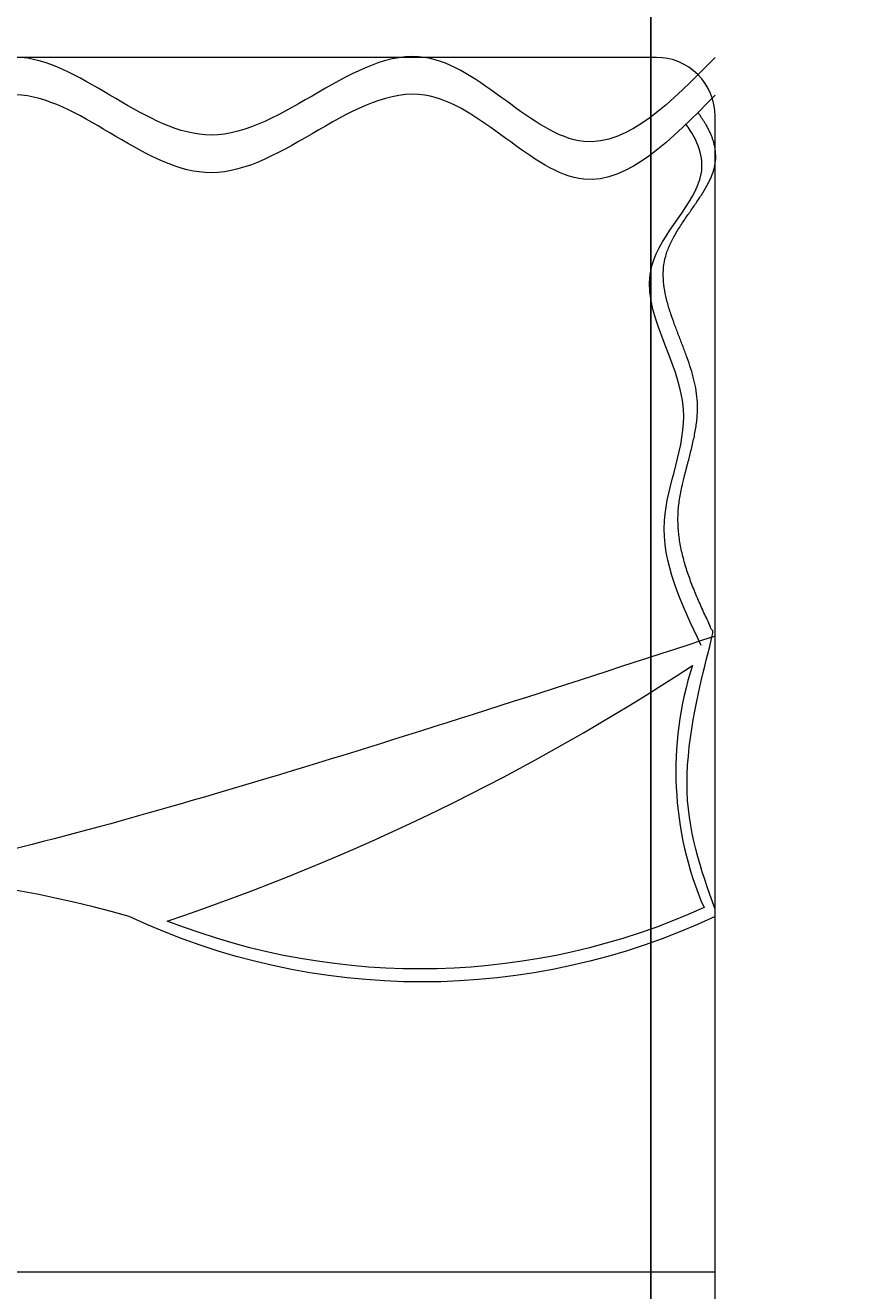
# Model space of a CAD drawing. Units: inches. Extents: x -61 to 1599, y -1316 to 257.
# Tile 53 of 204: x 143 to 192, y -408 to -334. Entities that reach past the tile are written whole.
import ezdxf

# ---------------------------------------------------------------- set-up
doc = ezdxf.new("R2010")
doc.units = ezdxf.units.IN
doc.header["$MEASUREMENT"] = 0
doc.layers.add('A-ANNO-DIMS', color=2, linetype='Continuous', lineweight=18)
doc.layers.add('FURNITURE', color=83, linetype='Continuous', lineweight=18)
doc.styles.get("Standard").update_dxf_attribs({"font": 'arial.ttf'})
doc.dimstyles.get("Standard").update_dxf_attribs({"dimtxt": 0.18, "dimasz": 0.18, "dimexe": 0.18, "dimexo": 0.0625, "dimgap": 0.09, "dimtad": 0, "dimtih": 1, "dimtoh": 1, "dimdec": 0, "dimzin": 0, "dimdsep": 46, "dimlunit": 3, "dimtxsty": 'Standard', "dimcen": 0.09, "dimadec": 0, "dimazin": 0, "dimtfac": 1, "dimtdec": 0, "dimtofl": 0, "dimtmove": 0, "dimatfit": 3, "dimfxl": 1, "dimtolj": 1, "dimtzin": 0, "dimarcsym": 0})

# ---------------------------------------------------------------- blocks, each defined once
blk = doc.blocks.new('BED-DOUBLE')
blk.add_line((1.272, 20.467), (70.263, 20.467))
for points in [[(1.272, 88.537), (1.272, 3.449, 0.414214), (4.722, 0), (66.813, 0, 0.414214), (70.263, 3.449), (70.263, 88.537, 0.414214), (66.813, 91.987), (4.722, 91.987, 0.414214)], [(38.01, 41.126, 0.064396), (68.933, 56.181, 0.181766), (69.614, 41.916, -0.202767)]]:
    blk.add_lwpolyline(points, format="xyb", close=True)
blk.add_lwpolyline([(70.263, 41.387, -0.22309), (35.767, 41.387, 0.142156), (1.272, 41.387)], format="xyb")
for points, knots in [([(70.263, 91.987), (67.707, 89.379), (62.206, 83.764), (52.487, 96.724), (40.92, 82.741), (28.609, 96.737), (15.695, 81.527), (6.205, 88.409), (1.272, 91.987)], [0, 0, 0, 0, 9.176033, 19.753992, 33.150145, 45.209422, 59.881559, 75.764594, 75.764594, 75.764594, 75.764594]), ([(70.263, 89.765), (67.707, 87.157), (62.206, 81.542), (52.487, 94.502), (40.92, 80.519), (28.609, 94.515), (15.695, 79.305), (6.205, 86.187), (1.272, 89.765)], [0, 0, 0, 0, 9.176033, 19.753992, 33.150145, 45.209422, 59.881559, 75.764594, 75.764594, 75.764594, 75.764594]), ([(69.451, 57.362), (68.289, 59.79), (66.113, 64.336), (70.043, 71.905), (64.118, 79.112), (70.314, 84.4), (69.244, 87.088), (68.552, 88.052)], [0, 0, 0, 0, 6.649676, 12.451782, 19.973966, 25.324174, 28.349676, 28.349676, 28.349676, 28.349676])]:
    blk.add_open_spline(points, degree=3, knots=knots)
for points, weights, knots in [([(70.263, 41.825), (68.018, 47.029), (68.018, 52.696), (70.263, 57.9), (69.1, 60.328), (66.924, 64.874), (70.854, 72.444), (64.929, 79.65), (71.186, 84.991), (70.014, 87.727), (69.253, 88.741)], [1, 0.945466318698, 0.945466318698, 1, 1, 1, 1, 1, 1, 1, 1], [0, 0, 0, 0, 0.814571, 0.814571, 0.814571, 7.464247, 13.266353, 20.788537, 26.138745, 29.321895, 29.321895, 29.321895, 29.321895]), ([(70.263, 57.9), (59.862, 50.943), (48.595, 45.5), (36.681, 41.677), (36.463, 41.771), (36.247, 41.868), (36.032, 41.966), (24.597, 45.284), (12.692, 45.258), (1.272, 41.889), (2.723, 44.9), (5.745, 51.172), (0.137, 60.702), (6.828, 69.972), (0.109, 77.787), (4.354, 84.383), (5.398, 86.876)], [1, 0.993520320424, 0.993520320424, 1, 0.99997444972, 0.99997444972, 1, 0.973174868659, 0.973174868659, 1, 1, 1, 1, 1, 1, 1, 1], [0, 0, 0, 0, 0.279074, 0.279074, 0.279074, 0.296584, 0.296584, 0.296584, 0.865868, 0.865868, 0.865868, 9.142578, 18.107734, 25.769226, 34.110801, 40.441511, 40.441511, 40.441511, 40.441511])]:
    blk.add_rational_spline(points, weights, degree=3, knots=knots)
blk = doc.blocks.new('*D687')
at = {"layer": 'A-ANNO-DIMS', "color": 0, "lineweight": -2, "transparency": 16777216}
for p, q in [((289.418, 181.677), (-61.077, 181.677)), ((-60.897, 181.497), (-60.897, -528.952)), ((-60.897, -1239.765), (-60.897, -529.316)), ((319.64, -1239.945), (-61.077, -1239.945))]:
    blk.add_line(p, q, dxfattribs=at)
at = {"layer": 'A-ANNO-DIMS', "color": 0, "transparency": 16777216}
for points in [[(-60.927, 181.497), (-60.867, 181.497), (-60.897, 181.677)], [(-60.927, -1239.765), (-60.867, -1239.765), (-60.897, -1239.945)]]:
    blk.add_solid(points, dxfattribs=at)
at = {"layer": 'DEFPOINTS', "color": 0, "transparency": 16777216}
for p in [(289.481, 181.677), (-60.897, -1239.945), (319.703, -1239.945)]:
    blk.add_point(p, dxfattribs=at)
at = {"layer": 'A-ANNO-DIMS', "color": 0, "transparency": 16777216, "insert": (-60.897, -529.134), "char_height": 0.18, "attachment_point": 5}
blk.add_mtext('\\A1;1421.6', dxfattribs=at)
blk = doc.blocks.new('*D699')
at = {"layer": 'A-ANNO-DIMS', "color": 0, "lineweight": -2, "transparency": 16777216}
for p, q in [((835.64, -167.169), (-61.077, -167.169)), ((-60.897, -167.349), (-60.897, -306.726)), ((-60.897, -446.466), (-60.897, -307.09)), ((841.64, -446.646), (-61.077, -446.646))]:
    blk.add_line(p, q, dxfattribs=at)
at = {"layer": 'A-ANNO-DIMS', "color": 0, "transparency": 16777216}
for points in [[(-60.927, -167.349), (-60.867, -167.349), (-60.897, -167.169)], [(-60.927, -446.466), (-60.867, -446.466), (-60.897, -446.646)]]:
    blk.add_solid(points, dxfattribs=at)
at = {"layer": 'DEFPOINTS', "color": 0, "transparency": 16777216}
for p in [(835.703, -167.169), (-60.897, -446.646), (841.703, -446.646)]:
    blk.add_point(p, dxfattribs=at)
at = {"layer": 'A-ANNO-DIMS', "color": 0, "transparency": 16777216, "insert": (-60.897, -306.908), "char_height": 0.18, "attachment_point": 5}
blk.add_mtext('\\A1;279.5', dxfattribs=at)
blk = doc.blocks.new('*D700')
at = {"layer": 'A-ANNO-DIMS', "color": 0, "lineweight": -2, "transparency": 16777216}
for p, q in [((14.703, -616.882), (14.703, 257.457)), ((14.883, 257.277), (96.772, 257.277)), ((179.572, 257.277), (97.683, 257.277)), ((179.752, -616.882), (179.752, 257.457))]:
    blk.add_line(p, q, dxfattribs=at)
at = {"layer": 'A-ANNO-DIMS', "color": 0, "transparency": 16777216}
for points in [[(14.883, 257.307), (14.883, 257.247), (14.703, 257.277)], [(179.572, 257.307), (179.572, 257.247), (179.752, 257.277)]]:
    blk.add_solid(points, dxfattribs=at)
at = {"layer": 'DEFPOINTS', "color": 0, "transparency": 16777216}
for p in [(179.752, 257.277), (14.703, -616.945), (179.752, -616.945)]:
    blk.add_point(p, dxfattribs=at)
at = {"layer": 'A-ANNO-DIMS', "color": 0, "transparency": 16777216, "insert": (97.227, 257.277), "char_height": 0.18, "attachment_point": 5}
blk.add_mtext('\\A1;165.05', dxfattribs=at)

msp = doc.modelspace()

# ---------------------------------------------------------------- block references
at = {"layer": 'FURNITURE'}
msp.add_blockref('BED-DOUBLE', (113.2612, -427.6961), dxfattribs=at)

# ---------------------------------------------------------------- dimensions: what is measured, and where the dimension line sits
at = {"layer": 'A-ANNO-DIMS'}
dim = msp.add_linear_dim(base=(179.7521, 257.2771), p1=(14.7028, -616.9446), p2=(179.7521, -616.9446), dimstyle='Standard', override={"dimdec": 2, "dimlfac": 1, "dimrnd": 0, "dimzin": 0, "dimdsep": 46, "dimlunit": 2}, dxfattribs=at)
dim.commit()
dim.dimension.update_dxf_attribs({"geometry": '*D700', "text_midpoint": (97.2274, 257.2771)})
for base, p1, p2, picture, middle in [((-60.8972, -1239.9446), (289.4807, 181.6771), (319.7028, -1239.9446), '*D687', (-60.8972, -529.1337)), ((-60.8972, -446.6462), (835.7028, -167.169), (841.7028, -446.6462), '*D699', (-60.8972, -306.9076))]:
    dim = msp.add_linear_dim(base=base, p1=p1, p2=p2, angle=90, dimstyle='Standard', override={"dimdec": 1, "dimlfac": 1, "dimrnd": 0, "dimzin": 0, "dimdsep": 46, "dimlunit": 2}, dxfattribs=at)
    dim.commit()
    dim.dimension.update_dxf_attribs({"geometry": picture, "text_midpoint": middle})

doc.saveas('drawing.dxf')
